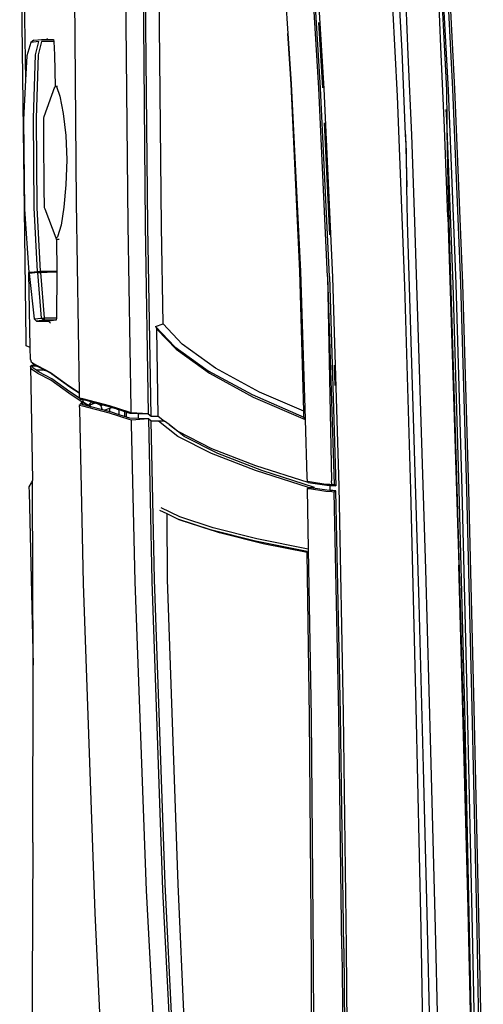
# Model space of a CAD drawing. Units: inches. Extents: x 22042254 to 25404563, y 17568978 to 17626777.
# Tile 27 of 45: x 22179811 to 22179827, y 17626261 to 17626295. Entities that reach past the tile are written whole.
import ezdxf

# ---------------------------------------------------------------- set-up
doc = ezdxf.new("R2010")
doc.units = ezdxf.units.IN
doc.header["$MEASUREMENT"] = 0
doc.layers.add('A-SITE-VEHI', color=8, linetype='Continuous', lineweight=18)
doc.layers.add('Edges', color=250, linetype='Continuous')

# ---------------------------------------------------------------- blocks, each defined once
blk = doc.blocks.new('Nissan Qashqai pl')
at = {"layer": 'Edges'}
for p, q in [((10.22184, 11.41141), (10.0431, 11.40746)), ((10.22178, 11.40944), (10.39472, 11.4128)), ((10.39471, 11.41477), (10.22184, 11.41141)), ((9.86732, 11.40312), (9.70104, 11.39829)), ((10.0431, 11.40746), (9.86732, 11.40312)), ((9.86732, 11.40115), (10.04305, 11.40549)), ((10.22152, 11.40604), (10.04287, 11.40208)), ((10.22157, 11.40372), (10.04288, 11.39976)), ((10.04305, 11.40549), (10.22178, 11.40944)), ((10.21754, 11.40282), (10.20433, 11.40249)), ((10.35645, 11.406), (10.21754, 11.40282)), ((10.39455, 11.40939), (10.22152, 11.40604)), ((10.3947, 11.40707), (10.22157, 11.40372)), ((9.70104, 11.39829), (9.54428, 11.39192)), ((9.54456, 11.38996), (9.70113, 11.39632)), ((9.64722, 11.38606), (9.92779, 11.39495)), ((9.70113, 11.39632), (9.86732, 11.40115)), ((9.86732, 11.39772), (9.70143, 11.39291)), ((9.86731, 11.39541), (9.70145, 11.39059)), ((9.85647, 11.39313), (9.97941, 11.39668)), ((10.04288, 11.39976), (9.86731, 11.39541)), ((10.04287, 11.40208), (9.86732, 11.39772)), ((10.07466, 11.39913), (9.92779, 11.39495)), ((9.97941, 11.39668), (10.09647, 11.39981)), ((10.20433, 11.40249), (10.07466, 11.39913)), ((10.09647, 11.39981), (10.09981, 11.39991)), ((10.09981, 11.39991), (10.20433, 11.40249)), ((9.54428, 11.39192), (9.47056, 11.38802)), ((9.47093, 11.38608), (9.54456, 11.38996)), ((9.70143, 11.39291), (9.54539, 11.3866)), ((9.70145, 11.39059), (9.56952, 11.38525)), ((9.62057, 11.38611), (9.67137, 11.38742)), ((9.67137, 11.38742), (9.85647, 11.39313)), ((9.51052, 11.38047), (9.46937, 11.37878)), ((9.472, 11.3812), (9.54539, 11.38506)), ((9.54539, 11.3866), (9.47204, 11.38275)), ((9.57554, 11.38341), (9.51052, 11.38047)), ((9.54539, 11.38506), (9.56952, 11.38525)), ((9.54543, 11.38483), (9.54539, 11.38506)), ((9.56952, 11.38525), (9.56093, 11.38491)), ((9.56952, 11.38525), (9.57857, 11.38532)), ((9.64722, 11.38606), (9.57554, 11.38341)), ((9.57857, 11.38532), (9.62057, 11.38611)), ((10.22011, 11.37591), (10.35861, 11.37907)), ((9.93119, 11.36807), (10.07764, 11.37224)), ((10.07764, 11.37224), (10.22011, 11.37591)), ((10.33528, 11.37248), (10.22032, 11.36991)), ((9.65144, 11.35922), (9.93119, 11.36807)), ((10.09097, 11.36665), (9.95835, 11.36298)), ((10.22109, 11.36462), (10.0423, 11.36067)), ((10.21909, 11.36987), (10.09097, 11.36665)), ((10.22022, 11.36991), (10.21909, 11.36987)), ((10.22022, 11.36991), (10.22032, 11.36991)), ((10.39547, 11.36796), (10.22109, 11.36462)), ((9.51676, 11.35387), (9.5812, 11.35675)), ((9.5812, 11.35675), (9.65144, 11.35922)), ((9.95835, 11.36298), (9.65101, 11.35355)), ((9.86731, 11.35632), (9.70295, 11.35156)), ((10.0423, 11.36067), (9.86731, 11.35632)), ((9.51403, 11.34924), (9.46047, 11.3465)), ((9.47609, 11.35222), (9.51676, 11.35387)), ((9.58112, 11.35216), (9.51403, 11.34924)), ((9.70295, 11.35156), (9.55025, 11.34551)), ((9.58112, 11.35216), (9.62312, 11.35314)), ((9.59402, 11.35272), (9.58112, 11.35216)), ((9.62312, 11.35314), (9.59402, 11.35272)), ((9.65101, 11.35355), (9.62312, 11.35314)), ((9.55025, 11.34551), (9.47817, 11.34178)), ((9.86438, 11.29822), (10.04724, 11.30183)), ((10.04757, 11.29962), (9.86806, 11.29595)), ((10.04724, 11.30183), (10.23568, 11.30434)), ((10.23666, 11.30223), (10.04757, 11.29962)), ((10.23693, 11.30084), (10.04769, 11.29822)), ((10.23568, 11.30434), (10.52995, 11.30682)), ((10.23666, 11.30223), (10.53508, 11.30497)), ((10.23693, 11.30084), (10.53477, 11.30357)), ((9.5443, 11.2863), (9.69599, 11.29318)), ((9.69529, 11.28925), (9.86302, 11.29443)), ((9.69529, 11.28925), (9.85984, 11.29245)), ((9.6954, 11.29067), (9.86406, 11.29586)), ((9.69599, 11.29318), (9.86438, 11.29822)), ((9.76686, 11.29454), (9.78322, 11.29505)), ((9.86285, 11.29254), (9.85984, 11.29245)), ((9.86275, 11.29093), (9.86285, 11.29254)), ((9.86285, 11.29254), (9.86302, 11.29443)), ((9.86406, 11.29586), (9.86302, 11.29443)), ((9.86368, 11.29096), (9.86383, 11.29336)), ((9.86383, 11.29336), (9.86406, 11.29586)), ((9.86783, 11.29345), (9.86768, 11.29105)), ((9.86806, 11.29595), (9.86783, 11.29345)), ((9.86806, 11.29595), (9.86905, 11.29456)), ((9.86887, 11.29269), (9.86857, 11.28791)), ((9.86905, 11.29456), (9.86887, 11.29269)), ((10.04769, 11.29822), (9.86905, 11.29456)), ((9.47391, 11.28204), (9.5443, 11.2863)), ((9.49097, 11.28193), (9.54338, 11.28517)), ((9.69529, 11.28925), (9.54369, 11.28221)), ((9.6954, 11.29067), (9.54381, 11.28364)), ((9.57172, 11.2865), (9.66181, 11.29073)), ((9.86052, 11.27457), (9.86255, 11.28779)), ((9.86149, 11.27538), (9.86353, 11.2886)), ((9.86255, 11.28779), (9.86275, 11.29093)), ((9.86275, 11.29093), (9.86368, 11.29096)), ((9.86353, 11.2886), (9.86368, 11.29096)), ((9.86368, 11.29096), (9.86434, 11.29098)), ((9.86434, 11.29098), (9.86768, 11.29105)), ((9.86753, 11.28868), (9.86549, 11.27544)), ((9.86857, 11.28791), (9.86653, 11.27467)), ((9.86768, 11.29105), (9.86753, 11.28868)), ((9.54369, 11.28221), (9.47347, 11.2779)), ((9.54381, 11.28364), (9.47359, 11.27933)), ((9.86521, 11.27876), (9.85155, 11.23625)), ((9.86521, 11.27376), (9.86521, 11.27876)), ((9.91486, 11.27364), (10.05053, 11.27601)), ((10.24533, 11.27621), (10.05014, 11.2747)), ((10.05053, 11.27601), (10.24534, 11.27774)), ((10.42923, 11.27673), (10.24533, 11.27621)), ((10.24534, 11.27774), (10.42889, 11.27835)), ((9.8039, 11.27002), (9.69119, 11.26675)), ((9.69131, 11.26744), (9.80992, 11.27113)), ((9.8039, 11.27002), (9.78845, 11.23427)), ((9.79049, 11.22834), (9.80869, 11.27016)), ((9.79253, 11.2294), (9.81069, 11.27115)), ((9.80869, 11.27016), (9.8039, 11.27002)), ((9.80992, 11.27113), (9.80869, 11.27016)), ((9.80992, 11.27113), (9.81069, 11.27115)), ((9.81069, 11.27115), (9.85734, 11.2726)), ((9.84753, 11.23118), (9.8611, 11.27338)), ((9.86521, 11.27376), (9.85155, 11.23125)), ((9.85734, 11.2726), (9.86034, 11.27269)), ((9.86034, 11.27269), (9.86052, 11.27457)), ((9.8611, 11.27338), (9.86034, 11.27269)), ((9.86121, 11.27348), (9.8611, 11.27338)), ((9.86121, 11.27348), (9.86149, 11.27538)), ((9.86521, 11.27354), (9.86653, 11.27467)), ((9.86524, 11.27376), (9.86521, 11.27376)), ((9.86524, 11.27376), (9.86521, 11.27354)), ((9.86521, 11.27354), (9.86636, 11.2728)), ((9.86549, 11.27544), (9.86524, 11.27376)), ((9.86653, 11.27467), (9.86636, 11.2728)), ((9.86636, 11.2728), (9.91486, 11.27364)), ((9.91486, 11.27364), (9.90657, 11.23225)), ((9.91688, 11.27275), (9.90857, 11.23128)), ((9.91767, 11.27277), (9.91057, 11.23732)), ((9.91767, 11.27277), (9.91688, 11.27275)), ((10.05014, 11.2747), (9.91767, 11.27277)), ((9.49969, 11.25726), (9.54029, 11.25996)), ((9.54029, 11.25996), (9.69131, 11.26744)), ((9.69119, 11.26675), (9.54041, 11.25978)), ((9.47103, 11.25536), (9.49969, 11.25726)), ((9.54041, 11.25978), (9.49969, 11.25726)), ((9.85155, 11.23625), (9.83784, 11.20068)), ((9.91057, 11.23732), (9.90181, 11.20207)), ((9.78845, 11.23427), (9.76924, 11.19888)), ((9.77129, 11.19294), (9.79049, 11.22834)), ((9.77333, 11.19399), (9.79253, 11.2294)), ((9.8338, 11.19559), (9.84753, 11.23118)), ((9.85155, 11.23125), (9.83784, 11.19568)), ((9.90657, 11.23225), (9.89779, 11.19698)), ((9.90857, 11.23128), (9.8998, 11.19602)), ((9.76924, 11.19888), (9.74989, 11.17207)), ((9.83784, 11.20068), (9.82412, 11.17361)), ((9.89779, 11.19698), (9.88907, 11.1701)), ((9.90181, 11.20207), (9.89309, 11.17519)), ((9.75194, 11.16612), (9.77129, 11.19294)), ((9.754, 11.16716), (9.77333, 11.19399)), ((9.82007, 11.16852), (9.8338, 11.19559)), ((9.83784, 11.19568), (9.82412, 11.16861)), ((9.89112, 11.16927), (9.8998, 11.19602)), ((10.50786, 11.1835), (10.18486, 11.16873)), ((9.82412, 11.17361), (9.81472, 11.16159)), ((9.89306, 11.17511), (9.89112, 11.16927)), ((9.89306, 11.17511), (9.89309, 11.17519)), ((10.50786, 11.17391), (10.18486, 11.15846)), ((9.74989, 11.17207), (9.73365, 11.15665)), ((9.73571, 11.15068), (9.75194, 11.16612)), ((9.73777, 11.15171), (9.754, 11.16716)), ((9.82412, 11.16861), (9.81187, 11.15294)), ((9.81472, 11.16159), (9.82007, 11.16852)), ((9.88907, 11.1701), (9.88181, 11.15507)), ((9.89108, 11.16915), (9.88666, 11.15997)), ((9.89112, 11.16927), (9.89108, 11.16915)), ((10.18486, 11.16873), (9.93935, 11.16021)), ((10.18944, 11.1563), (10.51094, 11.17209)), ((9.80783, 11.15283), (9.81187, 11.15794)), ((9.81467, 11.16159), (9.81187, 11.15794)), ((9.81187, 11.15794), (9.81187, 11.15294)), ((9.81472, 11.16159), (9.81467, 11.16159)), ((9.88666, 11.15997), (9.88383, 11.15407)), ((9.93935, 11.16021), (9.88666, 11.15997)), ((10.18486, 11.15846), (9.93935, 11.14974)), ((10.51126, 11.16029), (10.18995, 11.14332)), ((9.49361, 11.1538), (9.32247, 11.15308)), ((9.65517, 11.15538), (9.49361, 11.1538)), ((9.73365, 11.15665), (9.65517, 11.15538)), ((9.73571, 11.15068), (9.73365, 11.15665)), ((9.73571, 11.15068), (9.73777, 11.15171)), ((9.80783, 11.15283), (9.73777, 11.15171)), ((9.80783, 11.14706), (9.80783, 11.15283)), ((9.81187, 11.15294), (9.81187, 11.14718)), ((9.93935, 11.14974), (9.81187, 11.14718)), ((9.9411, 11.14751), (10.18944, 11.1563)), ((9.49361, 11.14285), (9.32247, 11.14209)), ((9.49218, 11.14085), (9.65398, 11.14234)), ((9.65517, 11.1445), (9.49361, 11.14285)), ((9.65398, 11.14234), (9.8061, 11.14474)), ((9.80783, 11.14706), (9.65517, 11.1445)), ((9.8061, 11.14474), (9.80507, 11.13091)), ((9.80579, 11.13689), (9.8061, 11.14474)), ((9.8061, 11.14474), (9.80783, 11.14706)), ((9.81013, 11.14486), (9.80984, 11.13689)), ((9.81013, 11.14486), (9.9411, 11.14751)), ((9.81187, 11.14718), (9.81013, 11.14486)), ((9.81013, 11.14486), (9.81122, 11.13108)), ((10.18995, 11.14332), (9.94142, 11.13412)), ((9.31979, 11.14026), (9.49218, 11.14085)), ((9.80551, 11.12983), (9.80579, 11.13689)), ((9.80984, 11.13689), (9.80579, 11.13689)), ((9.80984, 11.13689), (9.80958, 11.12996)), ((9.94142, 11.13412), (9.81425, 11.13118)), ((9.49192, 11.12689), (9.31945, 11.12622)), ((9.65381, 11.12845), (9.49192, 11.12689)), ((9.80203, 11.13089), (9.65381, 11.12845)), ((9.79917, 11.11333), (9.80444, 11.12904)), ((9.80507, 11.13091), (9.80203, 11.13089)), ((9.80261, 11.12117), (9.80409, 11.12559)), ((9.80409, 11.12559), (9.8045, 11.12682)), ((9.80409, 11.12559), (9.80814, 11.12561)), ((9.80444, 11.12904), (9.80507, 11.13091)), ((9.8045, 11.12682), (9.80459, 11.12708)), ((9.8045, 11.12682), (9.80854, 11.12682)), ((9.80459, 11.12708), (9.80551, 11.12983)), ((9.80862, 11.12708), (9.80459, 11.12708)), ((9.81061, 11.12921), (9.80538, 11.1135)), ((9.80814, 11.12561), (9.8067, 11.12126)), ((9.80854, 11.12682), (9.80814, 11.12561)), ((9.80862, 11.12708), (9.80854, 11.12682)), ((9.80958, 11.12996), (9.80862, 11.12708)), ((9.81122, 11.13108), (9.81061, 11.12921)), ((9.81425, 11.13118), (9.81122, 11.13108)), ((9.80078, 11.11568), (9.80143, 11.11762)), ((9.80302, 11.12118), (9.80143, 11.11762)), ((9.80143, 11.11762), (9.80261, 11.12117)), ((9.80302, 11.12118), (9.80261, 11.12117)), ((9.8067, 11.12126), (9.80302, 11.12118)), ((9.8067, 11.12126), (9.80436, 11.11419)), ((9.79366, 11.09176), (9.79917, 11.11333)), ((9.79869, 11.10799), (9.80024, 11.11406)), ((9.80538, 11.1135), (9.79986, 11.09192)), ((9.80024, 11.11406), (9.80078, 11.11568)), ((9.80145, 11.11385), (9.80078, 11.11568)), ((9.80428, 11.11385), (9.80145, 11.11385)), ((9.80311, 11.10927), (9.80145, 11.11385)), ((9.80428, 11.11385), (9.80311, 11.10927)), ((9.80436, 11.11419), (9.80428, 11.11385)), ((9.79636, 11.09882), (9.79729, 11.10234)), ((9.79729, 11.10234), (9.79774, 11.10424)), ((9.79774, 11.10331), (9.79729, 11.10234)), ((9.79729, 11.10234), (9.79774, 11.10111)), ((9.79867, 11.10531), (9.79774, 11.10331)), ((9.79774, 11.10424), (9.79779, 11.10443)), ((9.79774, 11.10424), (9.79774, 11.10331)), ((9.79779, 11.10443), (9.79869, 11.10799)), ((9.79867, 11.10531), (9.79779, 11.10443)), ((9.79923, 11.10651), (9.79867, 11.10531)), ((9.79923, 11.10651), (9.79869, 11.10799)), ((9.80273, 11.10778), (9.79923, 11.10651)), ((9.80273, 11.10778), (9.80033, 11.09835)), ((9.80311, 11.10927), (9.80273, 11.10778)), ((9.94259, 11.09232), (10.20814, 11.10172)), ((10.20814, 11.10172), (10.31203, 11.10643)), ((9.79636, 11.09882), (9.79429, 11.09068)), ((9.79923, 11.09659), (9.79628, 11.09185)), ((9.79636, 11.09882), (9.79923, 11.09659)), ((9.79642, 11.09173), (9.79963, 11.09662)), ((9.79774, 11.10111), (9.79774, 11.09979)), ((9.79774, 11.10111), (9.7985, 11.09903)), ((9.79774, 11.09979), (9.7985, 11.09903)), ((9.7985, 11.09903), (9.79886, 11.09803)), ((9.79984, 11.09644), (9.79885, 11.09252)), ((9.79886, 11.09803), (9.79984, 11.09757)), ((9.79984, 11.09757), (9.79923, 11.09659)), ((9.80025, 11.09803), (9.79963, 11.09662)), ((9.80008, 11.09735), (9.79963, 11.09662)), ((9.79963, 11.09662), (9.79984, 11.09644)), ((9.80033, 11.09835), (9.79984, 11.09757)), ((9.80008, 11.09735), (9.79984, 11.09644)), ((9.80025, 11.09803), (9.80008, 11.09735)), ((9.80033, 11.09835), (9.80025, 11.09803)), ((9.46731, 11.08523), (9.63583, 11.08663)), ((9.63583, 11.08663), (9.78874, 11.08892)), ((9.78318, 11.08047), (9.78874, 11.08892)), ((9.78422, 11.08144), (9.78911, 11.08892)), ((9.79335, 11.08923), (9.78833, 11.08154)), ((9.78874, 11.08892), (9.78911, 11.08892)), ((9.78911, 11.08892), (9.79002, 11.08894)), ((9.79655, 11.09153), (9.78937, 11.0806)), ((9.79002, 11.08894), (9.79309, 11.08897)), ((9.79309, 11.08897), (9.79344, 11.09065)), ((9.79309, 11.08897), (9.79335, 11.08923)), ((9.79335, 11.08923), (9.79413, 11.09005)), ((9.79344, 11.09065), (9.79366, 11.09176)), ((9.79344, 11.09065), (9.79376, 11.09037)), ((9.79413, 11.09005), (9.79429, 11.09068)), ((9.79549, 11.09252), (9.79429, 11.09068)), ((9.79628, 11.09185), (9.79549, 11.09252)), ((9.79628, 11.09185), (9.79626, 11.0918)), ((9.79642, 11.09173), (9.79628, 11.09185)), ((9.79639, 11.09168), (9.79642, 11.09173)), ((9.79665, 11.09153), (9.79642, 11.09173)), ((9.79655, 11.09153), (9.79665, 11.09153)), ((9.7983, 11.09006), (9.79655, 11.09153)), ((9.79665, 11.09153), (9.7986, 11.09159)), ((9.79767, 11.09066), (9.79665, 11.09153)), ((9.79824, 11.09018), (9.79767, 11.09066)), ((9.7986, 11.09159), (9.79824, 11.09018)), ((9.7983, 11.09006), (9.79824, 11.09018)), ((9.79862, 11.08979), (9.7983, 11.09006)), ((9.79885, 11.09252), (9.7986, 11.09159)), ((9.79862, 11.08979), (9.79928, 11.08913)), ((9.79986, 11.09192), (9.79928, 11.08913)), ((9.79928, 11.08913), (9.80235, 11.08924)), ((9.80235, 11.08924), (9.94259, 11.09232)), ((9.56409, 11.07604), (9.58178, 11.07816)), ((9.58178, 11.07816), (9.60156, 11.07911)), ((9.60156, 11.07911), (9.62147, 11.0782)), ((9.62147, 11.0782), (9.63954, 11.07656)), ((9.77275, 11.06605), (9.78318, 11.08047)), ((9.77376, 11.06705), (9.78422, 11.08144)), ((9.78833, 11.08154), (9.77778, 11.06711)), ((9.78937, 11.0806), (9.77881, 11.06614)), ((9.54224, 11.0706), (9.54217, 11.07161)), ((9.54224, 11.0706), (9.54241, 11.07066)), ((9.54231, 11.06958), (9.54224, 11.0706)), ((9.54241, 11.07066), (9.55026, 11.07357)), ((9.54255, 11.0695), (9.54241, 11.07066)), ((9.55026, 11.07357), (9.56409, 11.07604)), ((9.63954, 11.07656), (9.65397, 11.07443)), ((9.6645, 11.07045), (9.64129, 11.06157)), ((9.65397, 11.07443), (9.66334, 11.07154)), ((9.66334, 11.07154), (9.6645, 11.07045)), ((9.66552, 11.07084), (9.6645, 11.07045)), ((9.66552, 11.07285), (9.66552, 11.07084)), ((9.66552, 11.07084), (9.69109, 11.07091)), ((9.69109, 11.07091), (9.69199, 11.07091)), ((9.69114, 11.06453), (9.69109, 11.07091)), ((9.69199, 11.07091), (9.69204, 11.06454)), ((9.69199, 11.07091), (9.72869, 11.07078)), ((9.72869, 11.07078), (9.73053, 11.0704)), ((9.72878, 11.06094), (9.72869, 11.07078)), ((9.73053, 11.0704), (9.73128, 11.06438)), ((9.73053, 11.0704), (9.73063, 11.06072)), ((9.50366, 11.06354), (9.50447, 11.0628)), ((9.50441, 11.0586), (9.50447, 11.0628)), ((9.50447, 11.0628), (9.50454, 11.06827)), ((9.50454, 11.06827), (9.50627, 11.06871)), ((9.50627, 11.06871), (9.50615, 11.0586)), ((9.50627, 11.06871), (9.5168, 11.06905)), ((9.5168, 11.06905), (9.54231, 11.06958)), ((9.54255, 11.0695), (9.54231, 11.06958)), ((9.56666, 11.06086), (9.54255, 11.0695)), ((9.69115, 11.06309), (9.69114, 11.06453)), ((9.69205, 11.06311), (9.69115, 11.06309)), ((9.69119, 11.05771), (9.69115, 11.06309)), ((9.69204, 11.06454), (9.69205, 11.06311)), ((9.69205, 11.06311), (9.69209, 11.05779)), ((9.73304, 11.06599), (9.73128, 11.06438)), ((9.73137, 11.0547), (9.73128, 11.06438)), ((9.76745, 11.05568), (9.77275, 11.06605)), ((9.76844, 11.05669), (9.77174, 11.06312)), ((9.77174, 11.06312), (9.77073, 11.05935)), ((9.77174, 11.06312), (9.77376, 11.06705)), ((9.77778, 11.06711), (9.77242, 11.0568)), ((9.77881, 11.06614), (9.77343, 11.05581)), ((9.50516, 11.05238), (9.50441, 11.0586)), ((9.51679, 11.05372), (9.50612, 11.05641)), ((9.50612, 11.05641), (9.50687, 11.05011)), ((9.50615, 11.0586), (9.51675, 11.0559)), ((9.51675, 11.0559), (9.56787, 11.05428)), ((9.56784, 11.06044), (9.56666, 11.06086)), ((9.58458, 11.06059), (9.56784, 11.06044)), ((9.56787, 11.05428), (9.64004, 11.05493)), ((9.62365, 11.06094), (9.58458, 11.06059)), ((9.64002, 11.06109), (9.62365, 11.06094)), ((9.64129, 11.06157), (9.64002, 11.06109)), ((9.64004, 11.05493), (9.69119, 11.05771)), ((9.69125, 11.05557), (9.64009, 11.05279)), ((9.69125, 11.05557), (9.69119, 11.05771)), ((9.69196, 11.04989), (9.69125, 11.05557)), ((9.69209, 11.05779), (9.72878, 11.06094)), ((9.69215, 11.05565), (9.69209, 11.05779)), ((9.72885, 11.0588), (9.69215, 11.05565)), ((9.69215, 11.05565), (9.69302, 11.04862)), ((9.69215, 11.05565), (9.69216, 11.04991)), ((9.72885, 11.0588), (9.72878, 11.06094)), ((9.72878, 11.06094), (9.73063, 11.06072)), ((9.73063, 11.06072), (9.72885, 11.0588)), ((9.7296, 11.05274), (9.72885, 11.0588)), ((9.7296, 11.05274), (9.73137, 11.0547)), ((9.73063, 11.06072), (9.73137, 11.0547)), ((9.76483, 11.0513), (9.76643, 11.054)), ((9.76643, 11.054), (9.76745, 11.05568)), ((9.76645, 11.05372), (9.76643, 11.054)), ((9.76647, 11.05348), (9.76758, 11.05528)), ((9.76731, 11.05429), (9.76734, 11.05448)), ((9.76758, 11.0511), (9.76731, 11.05429)), ((9.76734, 11.05448), (9.76758, 11.05528)), ((9.76758, 11.05528), (9.76844, 11.05669)), ((9.76763, 11.05548), (9.76777, 11.056)), ((9.77123, 11.05496), (9.76904, 11.05158)), ((9.77343, 11.05581), (9.77004, 11.05057)), ((9.77073, 11.05935), (9.77091, 11.05485)), ((9.77091, 11.05485), (9.77123, 11.05496)), ((9.77242, 11.0568), (9.77123, 11.05496)), ((9.25173, 11.04109), (9.53716, 11.04591)), ((9.50516, 11.05238), (9.50687, 11.05011)), ((9.50687, 11.05011), (9.5176, 11.04694)), ((9.56793, 11.05214), (9.51679, 11.05372)), ((9.5176, 11.04694), (9.53716, 11.04591)), ((9.53716, 11.04591), (9.56889, 11.04424)), ((9.64009, 11.05279), (9.56793, 11.05214)), ((9.64105, 11.04501), (9.69213, 11.04852)), ((9.74656, 11.04638), (9.64105, 11.04501)), ((9.69216, 11.04991), (9.69196, 11.04989)), ((9.69213, 11.04852), (9.69196, 11.04989)), ((9.69216, 11.04991), (9.69213, 11.04852)), ((9.75265, 11.04954), (9.69213, 11.04852)), ((9.69302, 11.04862), (9.7296, 11.05274)), ((9.75114, 11.04628), (9.74656, 11.04638)), ((9.75265, 11.04954), (9.75114, 11.04628)), ((9.76234, 11.04971), (9.75265, 11.04954)), ((9.76234, 11.04971), (9.76425, 11.05042)), ((9.76425, 11.05042), (9.76523, 11.05144)), ((9.76425, 11.05042), (9.76477, 11.05127)), ((9.76477, 11.05127), (9.76483, 11.0513)), ((9.76523, 11.05144), (9.76647, 11.05348)), ((9.7667, 11.05081), (9.76647, 11.05348)), ((9.76758, 11.0511), (9.7667, 11.05081)), ((9.76769, 11.0498), (9.7667, 11.05081)), ((9.76904, 11.05158), (9.76758, 11.0511)), ((9.76774, 11.04981), (9.76769, 11.0498)), ((9.76774, 11.04981), (9.85978, 11.05135)), ((9.77004, 11.05057), (9.76774, 11.04981)), ((9.8643, 11.05143), (9.85978, 11.05135)), ((9.85978, 11.05135), (9.86144, 11.05043)), ((9.86144, 11.05043), (9.8647, 11.04853)), ((10.00853, 11.05192), (9.8643, 11.05143)), ((9.8647, 11.04853), (9.86899, 11.04876)), ((9.86899, 11.04876), (10.00853, 11.05192)), ((10.01239, 11.05193), (10.00853, 11.05192)), ((10.15127, 11.05172), (10.01239, 11.05193)), ((10.15127, 11.05172), (10.26766, 11.05118)), ((10.26766, 11.05118), (10.31893, 11.05108)), ((9.64105, 11.04501), (9.351, 11.04112)), ((9.56889, 11.04424), (9.64105, 11.04501))]:
    blk.add_line(p, q, dxfattribs=at)
blk = doc.blocks.new('CAR')
blk.add_blockref('Nissan Qashqai pl', (-9.74328, -11.91512))

msp = doc.modelspace()

# ---------------------------------------------------------------- block references
at = {"layer": 'A-SITE-VEHI', "xscale": 43.56002006885659, "yscale": 43.56002006885659, "zscale": 43.56002006885659, "rotation": 270}
msp.add_blockref('CAR', (22179848.861, 17626284.325), dxfattribs=at)

doc.saveas('drawing.dxf')
